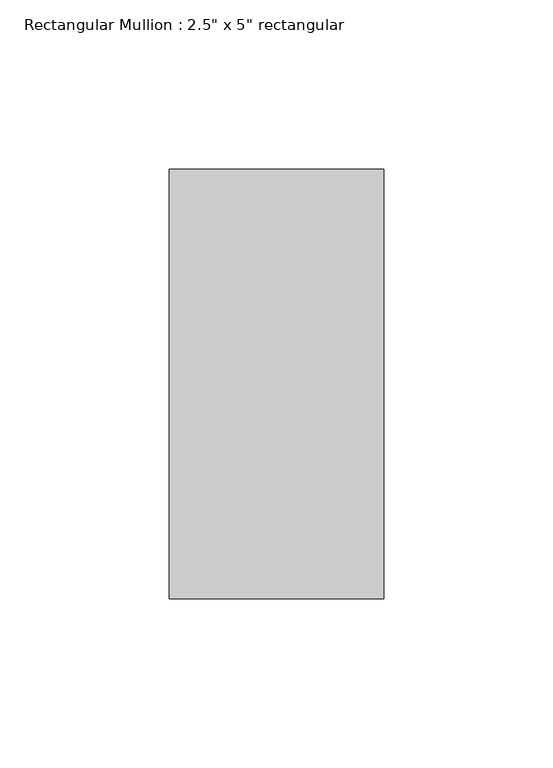
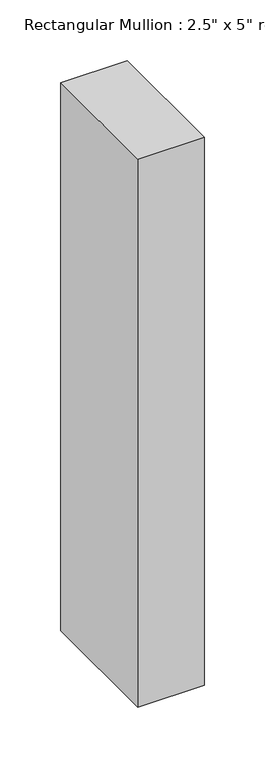
"""IFC4 building model written with IfcOpenShell, lengths in millimetres: member geometry."""

from ifc_helpers import new_model, si_unit, frame, origin, place, context, project, spatial, polyline, outline, extrude, source, transform, mapped, element, save


def member_73c075c8(model_context):
    return source(origin(), model_context, "Body", "SweptSolid", [
        extrude(outline(polyline([(0.0, 63.5), (0.0, -63.5), (-63.5, -63.5), (-63.5, 63.5), (0.0, 63.5)])), frame((0.0, 0.0, -552.45), z_axis=(0.0, 0.0, 1.0), x_axis=(1.0, 0.0, 0.0)), (0.0, 0.0, 1.0), 552.45),
    ])


if __name__ == "__main__":
    model = new_model("IFC4")
    model_context = context("Model", 3, world=origin())
    ifc_project = project(units=[si_unit("LENGTHUNIT", "METRE", prefix="MILLI")], contexts=[model_context])
    site = spatial("IfcSite", under=ifc_project)
    building = spatial("IfcBuilding", under=site)
    placement = place(None, origin())
    member_shape = member_73c075c8(model_context)
    element("IfcMember", 1, ObjectType="Rectangular Mullion : 2.5\" x 5\" rectangular", at=placement, inside=building, context=model_context, shape_type="MappedRepresentation", body=[
        mapped(member_shape, transform((0.0, 0.0, 0.0), x_axis=(1.0, 0.0, 0.0), y_axis=(0.0, 1.0, 0.0), z_axis=(0.0, 0.0, 1.0))),
    ])
    save(model, "model.ifc")

# Revit data of these elements
# Type "Rectangular Mullion : 2.5\" x 5\" rectangular"
#   built-in parameter 1007304 = 0.416667 (stored number, unit not read)
#   built-in parameter 1007301 = 0.104167 (stored number, unit not read)
#   built-in parameter 1007300 = 0.104167 (stored number, unit not read)
# Element 1 (IfcMember, "Rectangular Mullion : 2.5\" x 5\" rectangular")
#   Materials on its faces: "Aluminum"
# Materials
#   "Aluminum": class "Metal", colour RGB 247 247 247, transparency 0, Description = "Aluminum 6061", Cost = 0
